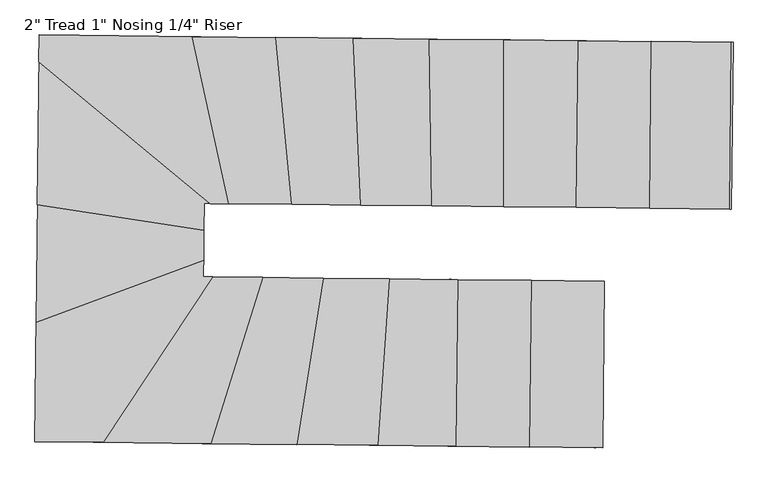
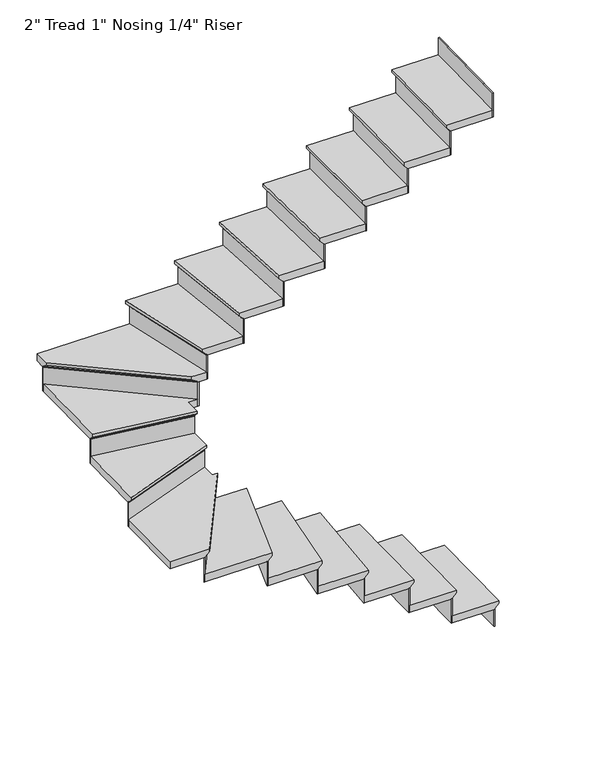
"""IFC4 building model written with IfcOpenShell, lengths in millimetres: stair flight geometry."""

from ifc_helpers import new_model, si_unit, origin, place, context, project, spatial, faceted_brep, source, transform, mapped, element, save


def stair_flight_e36c3716(model_context):
    return source(origin(), model_context, "Body", "Brep", [
        faceted_brep([(-1961.6349602, -4965.4067295, 9751.4833333), (-1961.6349602, -4965.4067295, 9770.5333333), (-1968.4523403, -5600.3701326, 9770.5333333), (-1968.4523403, -5600.3701326, 9751.4833333), (-1987.0334963, -4965.1340343, 9726.0833333), (-1993.8508764, -5600.0974374, 9726.0833333), (-2266.4173937, -4962.134387, 9770.5333333), (-2273.2347738, -5597.0977902, 9770.5333333), (-1993.8508764, -5600.0974374, 9719.7333333), (-2273.2347738, -5597.0977902, 9719.7333333), (-2266.4173937, -4962.134387, 9719.7333333), (-1987.0334963, -4965.1340343, 9719.7333333)], [[[0, 1, 2, 3]], [[4, 0, 3, 5]], [[2, 1, 6, 7]], [[8, 9, 10, 11]], [[2, 7, 9, 8, 5, 3]], [[8, 11, 4, 5]], [[6, 1, 0, 4, 11, 10]], [[7, 6, 10, 9]]]),
        faceted_brep([(-1987.0334963, -4965.1340343, 9719.7333333), (-1987.0334963, -4965.1340343, 9601.2), (-1993.3831304, -4965.0658605, 9601.2), (-1993.3831304, -4965.0658605, 9719.7333333), (-1993.8508764, -5600.0974374, 9719.7333333), (-2000.2005104, -5600.0292636, 9719.7333333), (-2000.2005104, -5600.0292636, 9601.2), (-1993.8508764, -5600.0974374, 9601.2)], [[[0, 1, 2, 3]], [[4, 5, 6, 7]], [[1, 0, 4, 7]], [[2, 1, 7, 6]], [[3, 2, 6, 5]], [[0, 3, 5, 4]]]),
        faceted_brep([(-2266.4173937, -4962.134387, 9889.0666667), (-2266.4173937, -4962.134387, 9719.7333333), (-2272.7670277, -4962.0662132, 9719.7333333), (-2272.7670277, -4962.0662132, 9889.0666667), (-2273.2347738, -5597.0977902, 9889.0666667), (-2279.5844078, -5597.0296164, 9889.0666667), (-2279.5844078, -5597.0296164, 9719.7333333), (-2273.2347738, -5597.0977902, 9719.7333333)], [[[0, 1, 2, 3]], [[4, 5, 6, 7]], [[1, 0, 4, 7]], [[2, 1, 7, 6]], [[3, 2, 6, 5]], [[0, 3, 5, 4]]]),
        faceted_brep([(-2247.8362377, -5597.3704854, 9939.8666667), (-2241.0188576, -4962.4070822, 9939.8666667), (-2545.8012911, -4959.1347398, 9939.8666667), (-2552.6186712, -5594.0981429, 9939.8666667), (-2273.2347738, -5597.0977902, 9889.0666667), (-2552.6186712, -5594.0981429, 9889.0666667), (-2545.8012911, -4959.1347398, 9889.0666667), (-2266.4173937, -4962.134387, 9889.0666667), (-2273.2347738, -5597.0977902, 9895.4166667), (-2247.8362377, -5597.3704854, 9920.8166667), (-2266.4173937, -4962.134387, 9895.4166667), (-2241.0188576, -4962.4070822, 9920.8166667)], [[[0, 1, 2, 3]], [[4, 5, 6, 7]], [[0, 3, 5, 4, 8, 9]], [[4, 7, 10, 8]], [[2, 1, 11, 10, 7, 6]], [[3, 2, 6, 5]], [[11, 1, 0, 9]], [[10, 11, 9, 8]]]),
        faceted_brep([(-2545.8012911, -4959.1347398, 10058.4), (-2545.8012911, -4959.1347398, 9889.0666667), (-2552.1509251, -4959.066566, 9889.0666667), (-2552.1509251, -4959.066566, 10058.4), (-2552.6186712, -5594.0981429, 10058.4), (-2558.9683052, -5594.0299691, 10058.4), (-2558.9683052, -5594.0299691, 9889.0666667), (-2552.6186712, -5594.0981429, 9889.0666667)], [[[0, 1, 2, 3]], [[4, 5, 6, 7]], [[1, 0, 4, 7]], [[2, 1, 7, 6]], [[3, 2, 6, 5]], [[0, 3, 5, 4]]]),
        faceted_brep([(-2527.2201351, -5594.3708381, 10109.2), (-2520.402755, -4959.407435, 10109.2), (-2806.7760852, -4956.3327447, 10109.2), (-2850.4973934, -5590.8999232, 10109.2), (-2552.6186712, -5594.0981429, 10058.4), (-2850.4973934, -5590.8999232, 10058.4), (-2806.7760852, -4956.3327447, 10058.4), (-2545.8012911, -4959.1347398, 10058.4), (-2552.6186712, -5594.0981429, 10064.75), (-2527.2201351, -5594.3708381, 10090.15), (-2545.8012911, -4959.1347398, 10064.75), (-2520.402755, -4959.407435, 10090.15)], [[[0, 1, 2, 3]], [[4, 5, 6, 7]], [[0, 3, 5, 4, 8, 9]], [[4, 7, 10, 8]], [[2, 1, 11, 10, 7, 6]], [[3, 2, 6, 5]], [[11, 1, 0, 9]], [[10, 11, 9, 8]]]),
        faceted_brep([(-2806.7760852, -4956.3327447, 10227.7333333), (-2806.7760852, -4956.3327447, 10058.4), (-2813.1364345, -4956.2644558, 10058.4), (-2813.1364345, -4956.2644558, 10227.7333333), (-2850.4973934, -5590.8999232, 10227.7333333), (-2856.8577426, -5590.8316344, 10227.7333333), (-2856.8577426, -5590.8316344, 10058.4), (-2850.4973934, -5590.8999232, 10058.4)], [[[0, 1, 2, 3]], [[4, 5, 6, 7]], [[1, 0, 4, 7]], [[2, 1, 7, 6]], [[3, 2, 6, 5]], [[0, 3, 5, 4]]]),
        faceted_brep([(-2825.0559965, -5591.1730786, 10278.5333333), (-2781.3346883, -4956.6059001, 10278.5333333), (-3058.0757112, -4953.6346284, 10278.5333333), (-3158.4280189, -5587.5937798, 10278.5333333), (-2850.4973934, -5590.8999232, 10227.7333333), (-3158.4280189, -5587.5937798, 10227.7333333), (-3058.0757112, -4953.6346284, 10227.7333333), (-2806.7760852, -4956.3327447, 10227.7333333), (-2850.4973934, -5590.8999232, 10234.0833333), (-2825.0559965, -5591.1730786, 10259.4833333), (-2806.7760852, -4956.3327447, 10234.0833333), (-2781.3346883, -4956.6059001, 10259.4833333)], [[[0, 1, 2, 3]], [[4, 5, 6, 7]], [[0, 3, 5, 4, 8, 9]], [[4, 7, 10, 8]], [[2, 1, 11, 10, 7, 6]], [[3, 2, 6, 5]], [[11, 1, 0, 9]], [[10, 11, 9, 8]]]),
        faceted_brep([(-3058.0757112, -4953.6346284, 10397.0666667), (-3058.0757112, -4953.6346284, 10227.7333333), (-3064.4938676, -4953.5657189, 10227.7333333), (-3064.4938676, -4953.5657189, 10397.0666667), (-3158.4280189, -5587.5937798, 10397.0666667), (-3164.8461752, -5587.5248703, 10397.0666667), (-3164.8461752, -5587.5248703, 10227.7333333), (-3158.4280189, -5587.5937798, 10227.7333333)], [[[0, 1, 2, 3]], [[4, 5, 6, 7]], [[1, 0, 4, 7]], [[2, 1, 7, 6]], [[3, 2, 6, 5]], [[0, 3, 5, 4]]]),
        faceted_brep([(-3132.7553936, -5587.8694178, 10447.8666667), (-3032.4030859, -4953.9102664, 10447.8666667), (-3289.3424431, -4951.1515984, 10447.8666667), (-3487.6403792, -5584.0591417, 10447.8666667), (-3158.4280189, -5587.5937798, 10397.0666667), (-3487.6403792, -5584.0591417, 10397.0666667), (-3289.3424431, -4951.1515984, 10397.0666667), (-3058.0757112, -4953.6346284, 10397.0666667), (-3158.4280189, -5587.5937798, 10403.4166667), (-3132.7553936, -5587.8694178, 10428.8166667), (-3058.0757112, -4953.6346284, 10403.4166667), (-3032.4030859, -4953.9102664, 10428.8166667)], [[[0, 1, 2, 3]], [[4, 5, 6, 7]], [[0, 3, 5, 4, 8, 9]], [[4, 7, 10, 8]], [[2, 1, 11, 10, 7, 6]], [[3, 2, 6, 5]], [[11, 1, 0, 9]], [[10, 11, 9, 8]]]),
        faceted_brep([(-3289.3424431, -4951.1515984, 10566.4), (-3289.3424431, -4951.1515984, 10397.0666667), (-3295.9745116, -4951.0803922, 10397.0666667), (-3295.9745116, -4951.0803922, 10566.4), (-3487.6403792, -5584.0591417, 10566.4), (-3494.2724477, -5583.9879355, 10566.4), (-3494.2724477, -5583.9879355, 10397.0666667), (-3487.6403792, -5584.0591417, 10397.0666667)], [[[0, 1, 2, 3]], [[4, 5, 6, 7]], [[1, 0, 4, 7]], [[2, 1, 7, 6]], [[3, 2, 6, 5]], [[0, 3, 5, 4]]]),
        faceted_brep([(-3461.1121052, -5584.3439665, 10617.2), (-3262.8141691, -4951.4364232, 10617.2), (-3484.2219113, -4949.0592457, 10617.2), (-3900.4163626, -5579.6273103, 10617.2), (-3487.6403792, -5584.0591417, 10566.4), (-3900.4163626, -5579.6273103, 10566.4), (-3484.2219113, -4949.0592457, 10566.4), (-3289.3424431, -4951.1515984, 10566.4), (-3487.6403792, -5584.0591417, 10572.75), (-3461.1121052, -5584.3439665, 10598.15), (-3289.3424431, -4951.1515984, 10572.75), (-3262.8141691, -4951.4364232, 10598.15)], [[[0, 1, 2, 3]], [[4, 5, 6, 7]], [[0, 3, 5, 4, 8, 9]], [[4, 7, 10, 8]], [[2, 1, 11, 10, 7, 6]], [[3, 2, 6, 5]], [[11, 1, 0, 9]], [[10, 11, 9, 8]]]),
        faceted_brep([(-3484.2219113, -4949.0592457, 10735.7333333), (-3484.2219113, -4949.0592457, 10566.4), (-3491.7768309, -4948.9781311, 10566.4), (-3491.7768309, -4948.9781311, 10735.7333333), (-3900.4163626, -5579.6273103, 10735.7333333), (-3907.9712823, -5579.5461958, 10735.7333333), (-3907.9712823, -5579.5461958, 10566.4), (-3900.4163626, -5579.6273103, 10566.4)], [[[0, 1, 2, 3]], [[4, 5, 6, 7]], [[1, 0, 4, 7]], [[2, 1, 7, 6]], [[3, 2, 6, 5]], [[0, 3, 5, 4]]]),
        faceted_brep([(-4125.8898698, -5095.6676694, 10786.5333333), (-4131.0593878, -5577.1509768, 10786.5333333), (-3870.196684, -5579.9517684, 10786.5333333), (-3454.0022327, -4949.3837038, 10786.5333333), (-3489.2786045, -4949.0049537, 10786.5333333), (-3488.312708, -4859.0423992, 10786.5333333), (-4131.0593878, -5577.1509768, 10735.7333333), (-4125.8898698, -5095.6676694, 10735.7333333), (-3488.312708, -4859.0423992, 10735.7333333), (-3489.2786045, -4949.0049537, 10735.7333333), (-3484.2219113, -4949.0592457, 10735.7333333), (-3900.4163626, -5579.6273103, 10735.7333333), (-3900.4163626, -5579.6273103, 10742.0833333), (-3870.196684, -5579.9517684, 10767.4833333), (-3484.2219113, -4949.0592457, 10742.0833333), (-3454.0022327, -4949.3837038, 10767.4833333)], [[[0, 1, 2, 3, 4, 5]], [[6, 7, 8, 9, 10, 11]], [[1, 0, 7, 6]], [[2, 1, 6, 11, 12, 13]], [[11, 10, 14, 12]], [[4, 3, 15, 14, 10, 9]], [[5, 4, 9, 8]], [[0, 5, 8, 7]], [[15, 3, 2, 13]], [[14, 15, 13, 12]]]),
        faceted_brep([(-3488.312708, -4859.0423992, 10905.0666667), (-3488.312708, -4859.0423992, 10735.7333333), (-3488.2396954, -4852.2420842, 10735.7333333), (-3488.2396954, -4852.2420842, 10905.0666667), (-4125.8898698, -5095.6676694, 10905.0666667), (-4125.8168572, -5088.8673543, 10905.0666667), (-4125.8168572, -5088.8673543, 10735.7333333), (-4125.8898698, -5095.6676694, 10735.7333333)], [[[0, 1, 2, 3]], [[4, 5, 6, 7]], [[1, 0, 4, 7]], [[2, 1, 7, 6]], [[3, 2, 6, 5]], [[0, 3, 5, 4]]]),
        faceted_brep([(-4126.1819202, -5122.8689296, 10955.8666667), (-3488.6047585, -4886.2436594, 10955.8666667), (-3487.1016265, -4746.243576, 10955.8666667), (-4121.0934321, -4648.9326558, 10955.8666667), (-4125.8898698, -5095.6676694, 10905.0666667), (-4121.0934321, -4648.9326558, 10905.0666667), (-3487.1016265, -4746.243576, 10905.0666667), (-3488.312708, -4859.0423992, 10905.0666667), (-4125.8898698, -5095.6676694, 10911.4166667), (-4126.1819202, -5122.8689296, 10936.8166667), (-3488.312708, -4859.0423992, 10911.4166667), (-3488.6047585, -4886.2436594, 10936.8166667)], [[[0, 1, 2, 3]], [[4, 5, 6, 7]], [[0, 3, 5, 4, 8, 9]], [[4, 7, 10, 8]], [[3, 2, 6, 5]], [[11, 1, 0, 9]], [[10, 11, 9, 8]], [[2, 1, 11, 10, 7, 6]]]),
        faceted_brep([(-3487.1016265, -4746.243576, 11074.4), (-3487.1016265, -4746.243576, 10905.0666667), (-3487.0327638, -4739.8297815, 10905.0666667), (-3487.0327638, -4739.8297815, 11074.4), (-4121.0934321, -4648.9326558, 11074.4), (-4121.0245695, -4642.5188612, 11074.4), (-4121.0245695, -4642.5188612, 10905.0666667), (-4121.0934321, -4648.9326558, 10905.0666667)], [[[0, 1, 2, 3]], [[4, 5, 6, 7]], [[1, 0, 4, 7]], [[2, 1, 7, 6]], [[3, 2, 6, 5]], [[0, 3, 5, 4]]]),
        faceted_brep([(-4121.3688828, -4674.587834, 11125.2), (-3487.3770772, -4771.8987542, 11125.2), (-3486.2789573, -4669.6210563, 11125.2), (-3423.6180491, -4670.2938246, 11125.2), (-4115.1699262, -4097.2237198, 11125.2), (-4121.0934321, -4648.9326558, 11074.4), (-4115.1699262, -4097.2237198, 11074.4), (-3423.6180491, -4670.2938246, 11074.4), (-3486.2789573, -4669.6210563, 11074.4), (-3487.1016265, -4746.243576, 11074.4), (-4121.0934321, -4648.9326558, 11080.75), (-4121.3688828, -4674.587834, 11106.15), (-3487.1016265, -4746.243576, 11080.75), (-3487.3770772, -4771.8987542, 11106.15)], [[[0, 1, 2, 3, 4]], [[5, 6, 7, 8, 9]], [[0, 4, 6, 5, 10, 11]], [[5, 9, 12, 10]], [[2, 1, 13, 12, 9, 8]], [[4, 3, 7, 6]], [[13, 1, 0, 11]], [[12, 13, 11, 10]], [[3, 2, 8, 7]]]),
        faceted_brep([(-3423.6180491, -4670.2938246, 11243.7333333), (-3423.6180491, -4670.2938246, 11074.4), (-3413.5354356, -4670.4020781, 11074.4), (-3413.5354356, -4670.4020781, 11243.7333333), (-4115.1699262, -4097.2237198, 11243.7333333), (-4115.0821626, -4089.0495147, 11243.7333333), (-4115.0821626, -4089.0495147, 11074.4), (-4115.1699262, -4097.2237198, 11074.4)], [[[0, 1, 2, 3]], [[4, 5, 6, 7]], [[1, 0, 4, 7]], [[2, 1, 7, 6]], [[3, 2, 6, 5]], [[0, 3, 5, 4]]]),
        faceted_brep([(-3506.4342514, -4034.368057, 11294.5333333), (-4114.4249804, -4027.8402731, 11294.5333333), (-4115.5209805, -4129.9205399, 11294.5333333), (-3463.9485035, -4669.8608106, 11294.5333333), (-3365.8789969, -4670.9137486, 11294.5333333), (-4114.4249804, -4027.8402731, 11243.7333333), (-3506.4342514, -4034.368057, 11243.7333333), (-3365.8789969, -4670.9137486, 11243.7333333), (-3423.6180491, -4670.2938246, 11243.7333333), (-4115.1699262, -4097.2237198, 11243.7333333), (-3423.6180491, -4670.2938246, 11250.0833333), (-4115.1699262, -4097.2237198, 11250.0833333), (-3463.9485035, -4669.8608106, 11275.4833333), (-4115.5209805, -4129.9205399, 11275.4833333)], [[[0, 1, 2, 3, 4]], [[5, 6, 7, 8, 9]], [[1, 0, 6, 5]], [[9, 8, 10, 11]], [[4, 3, 12, 10, 8, 7]], [[0, 4, 7, 6]], [[12, 3, 2, 13]], [[10, 12, 13, 11]], [[2, 1, 5, 9, 11, 13]]]),
        faceted_brep([(-3365.8789969, -4670.9137486, 11413.0666667), (-3365.8789969, -4670.9137486, 11243.7333333), (-3359.3605829, -4670.9837346, 11243.7333333), (-3359.3605829, -4670.9837346, 11413.0666667), (-3506.4342514, -4034.368057, 11413.0666667), (-3499.9158374, -4034.438043, 11413.0666667), (-3499.9158374, -4034.438043, 11243.7333333), (-3506.4342514, -4034.368057, 11243.7333333)], [[[0, 1, 2, 3]], [[4, 5, 6, 7]], [[1, 0, 4, 7]], [[2, 1, 7, 6]], [[3, 2, 6, 5]], [[0, 3, 5, 4]]]),
        faceted_brep([(-3532.5079076, -4034.0881133, 11463.8666667), (-3391.9526531, -4670.6338049, 11463.8666667), (-3127.2086135, -4673.4762691, 11463.8666667), (-3187.4049598, -4037.793363, 11463.8666667), (-3506.4342514, -4034.368057, 11413.0666667), (-3187.4049598, -4037.793363, 11413.0666667), (-3127.2086135, -4673.4762691, 11413.0666667), (-3365.8789969, -4670.9137486, 11413.0666667), (-3506.4342514, -4034.368057, 11419.4166667), (-3532.5079076, -4034.0881133, 11444.8166667), (-3365.8789969, -4670.9137486, 11419.4166667), (-3391.9526531, -4670.6338049, 11444.8166667)], [[[0, 1, 2, 3]], [[4, 5, 6, 7]], [[0, 3, 5, 4, 8, 9]], [[4, 7, 10, 8]], [[2, 1, 11, 10, 7, 6]], [[3, 2, 6, 5]], [[11, 1, 0, 9]], [[10, 11, 9, 8]]]),
        faceted_brep([(-3127.2086135, -4673.4762691, 11582.4), (-3127.2086135, -4673.4762691, 11413.0666667), (-3120.8237144, -4673.5448215, 11413.0666667), (-3120.8237144, -4673.5448215, 11582.4), (-3187.4049598, -4037.793363, 11582.4), (-3181.0200608, -4037.8619154, 11582.4), (-3181.0200608, -4037.8619154, 11413.0666667), (-3187.4049598, -4037.793363, 11413.0666667)], [[[0, 1, 2, 3]], [[4, 5, 6, 7]], [[1, 0, 4, 7]], [[2, 1, 7, 6]], [[3, 2, 6, 5]], [[0, 3, 5, 4]]]),
        faceted_brep([(-3212.9445562, -4037.5191533, 11633.2), (-3152.7482098, -4673.2020594, 11633.2), (-2863.8799111, -4676.3035373, 11633.2), (-2892.1704009, -4040.9631932, 11633.2), (-3187.4049598, -4037.793363, 11582.4), (-2892.1704009, -4040.9631932, 11582.4), (-2863.8799111, -4676.3035373, 11582.4), (-3127.2086135, -4673.4762691, 11582.4), (-3187.4049598, -4037.793363, 11588.75), (-3212.9445562, -4037.5191533, 11614.15), (-3127.2086135, -4673.4762691, 11588.75), (-3152.7482098, -4673.2020594, 11614.15)], [[[0, 1, 2, 3]], [[4, 5, 6, 7]], [[0, 3, 5, 4, 8, 9]], [[4, 7, 10, 8]], [[2, 1, 11, 10, 7, 6]], [[3, 2, 6, 5]], [[11, 1, 0, 9]], [[10, 11, 9, 8]]]),
        faceted_brep([(-2863.8799111, -4676.3035373, 11751.7333333), (-2863.8799111, -4676.3035373, 11582.4), (-2857.5205787, -4676.3718152, 11582.4), (-2857.5205787, -4676.3718152, 11751.7333333), (-2892.1704009, -4040.9631932, 11751.7333333), (-2885.8110685, -4041.0314712, 11751.7333333), (-2885.8110685, -4041.0314712, 11582.4), (-2892.1704009, -4040.9631932, 11582.4)], [[[0, 1, 2, 3]], [[4, 5, 6, 7]], [[1, 0, 4, 7]], [[2, 1, 7, 6]], [[3, 2, 6, 5]], [[0, 3, 5, 4]]]),
        faceted_brep([(-2917.6077305, -4040.6900815, 11802.5333333), (-2889.3172407, -4676.0304256, 11802.5333333), (-2593.0867697, -4679.2109486, 11802.5333333), (-2604.2529652, -4044.0544621, 11802.5333333), (-2892.1704009, -4040.9631932, 11751.7333333), (-2604.2529652, -4044.0544621, 11751.7333333), (-2593.0867697, -4679.2109486, 11751.7333333), (-2863.8799111, -4676.3035373, 11751.7333333), (-2892.1704009, -4040.9631932, 11758.0833333), (-2917.6077305, -4040.6900815, 11783.4833333), (-2863.8799111, -4676.3035373, 11758.0833333), (-2889.3172407, -4676.0304256, 11783.4833333)], [[[0, 1, 2, 3]], [[4, 5, 6, 7]], [[0, 3, 5, 4, 8, 9]], [[4, 7, 10, 8]], [[2, 1, 11, 10, 7, 6]], [[3, 2, 6, 5]], [[11, 1, 0, 9]], [[10, 11, 9, 8]]]),
        faceted_brep([(-2593.0867697, -4679.2109486, 11921.0666667), (-2593.0867697, -4679.2109486, 11751.7333333), (-2586.7345895, -4679.2791497, 11751.7333333), (-2586.7345895, -4679.2791497, 11921.0666667), (-2604.2529652, -4044.0544621, 11921.0666667), (-2597.900785, -4044.1226632, 11921.0666667), (-2597.900785, -4044.1226632, 11751.7333333), (-2604.2529652, -4044.0544621, 11751.7333333)], [[[0, 1, 2, 3]], [[4, 5, 6, 7]], [[1, 0, 4, 7]], [[2, 1, 7, 6]], [[3, 2, 6, 5]], [[0, 3, 5, 4]]]),
        faceted_brep([(-2629.661686, -4043.7816575, 11971.8666667), (-2618.4954904, -4678.9381441, 11971.8666667), (-2319.0528449, -4682.1531551, 11971.8666667), (-2319.536107, -4047.1113675, 11971.8666667), (-2604.2529652, -4044.0544621, 11921.0666667), (-2319.536107, -4047.1113675, 11921.0666667), (-2319.0528449, -4682.1531551, 11921.0666667), (-2593.0867697, -4679.2109486, 11921.0666667), (-2604.2529652, -4044.0544621, 11927.4166667), (-2629.661686, -4043.7816575, 11952.8166667), (-2593.0867697, -4679.2109486, 11927.4166667), (-2618.4954904, -4678.9381441, 11952.8166667)], [[[0, 1, 2, 3]], [[4, 5, 6, 7]], [[0, 3, 5, 4, 8, 9]], [[4, 7, 10, 8]], [[2, 1, 11, 10, 7, 6]], [[3, 2, 6, 5]], [[11, 1, 0, 9]], [[10, 11, 9, 8]]]),
        faceted_brep([(-2319.0528449, -4682.1531551, 12090.4), (-2319.0528449, -4682.1531551, 11921.0666667), (-2312.7027912, -4682.2213334, 11921.0666667), (-2312.7027912, -4682.2213334, 12090.4), (-2319.536107, -4047.1113675, 12090.4), (-2313.1860533, -4047.1795458, 12090.4), (-2313.1860533, -4047.1795458, 11921.0666667), (-2319.536107, -4047.1113675, 11921.0666667)], [[[0, 1, 2, 3]], [[4, 5, 6, 7]], [[1, 0, 4, 7]], [[2, 1, 7, 6]], [[3, 2, 6, 5]], [[0, 3, 5, 4]]]),
        faceted_brep([(-2344.9363219, -4046.8386542, 12141.2), (-2344.4530598, -4681.8804418, 12141.2), (-2043.3209474, -4685.113592, 12141.2), (-2036.5035673, -4050.1501889, 12141.2), (-2319.536107, -4047.1113675, 12090.4), (-2036.5035673, -4050.1501889, 12090.4), (-2043.3209474, -4685.113592, 12090.4), (-2319.0528449, -4682.1531551, 12090.4), (-2319.536107, -4047.1113675, 12096.75), (-2344.9363219, -4046.8386542, 12122.15), (-2319.0528449, -4682.1531551, 12096.75), (-2344.4530598, -4681.8804418, 12122.15)], [[[0, 1, 2, 3]], [[4, 5, 6, 7]], [[0, 3, 5, 4, 8, 9]], [[4, 7, 10, 8]], [[2, 1, 11, 10, 7, 6]], [[3, 2, 6, 5]], [[11, 1, 0, 9]], [[10, 11, 9, 8]]]),
        faceted_brep([(-2043.3209474, -4685.113592, 12259.7333333), (-2043.3209474, -4685.113592, 12090.4), (-2036.9713133, -4685.1817658, 12090.4), (-2036.9713133, -4685.1817658, 12259.7333333), (-2036.5035673, -4050.1501889, 12259.7333333), (-2030.1539332, -4050.2183627, 12259.7333333), (-2030.1539332, -4050.2183627, 12090.4), (-2036.5035673, -4050.1501889, 12090.4)], [[[0, 1, 2, 3]], [[4, 5, 6, 7]], [[1, 0, 4, 7]], [[2, 1, 7, 6]], [[3, 2, 6, 5]], [[0, 3, 5, 4]]]),
        faceted_brep([(-2061.9021034, -4049.8774937, 12310.5333333), (-2068.7194835, -4684.8408968, 12310.5333333), (-1763.93705, -4688.1132393, 12310.5333333), (-1757.1196699, -4053.1498361, 12310.5333333), (-2036.5035673, -4050.1501889, 12259.7333333), (-1757.1196699, -4053.1498361, 12259.7333333), (-1763.93705, -4688.1132393, 12259.7333333), (-2043.3209474, -4685.113592, 12259.7333333), (-2036.5035673, -4050.1501889, 12266.0833333), (-2061.9021034, -4049.8774937, 12291.4833333), (-2043.3209474, -4685.113592, 12266.0833333), (-2068.7194835, -4684.8408968, 12291.4833333)], [[[0, 1, 2, 3]], [[4, 5, 6, 7]], [[0, 3, 5, 4, 8, 9]], [[4, 7, 10, 8]], [[2, 1, 11, 10, 7, 6]], [[3, 2, 6, 5]], [[11, 1, 0, 9]], [[10, 11, 9, 8]]]),
        faceted_brep([(-1763.93705, -4688.1132393, 12429.0666667), (-1763.93705, -4688.1132393, 12259.7333333), (-1757.5874159, -4688.1814131, 12259.7333333), (-1757.5874159, -4688.1814131, 12429.0666667), (-1757.1196699, -4053.1498361, 12429.0666667), (-1750.7700359, -4053.2180099, 12429.0666667), (-1750.7700359, -4053.2180099, 12259.7333333), (-1757.1196699, -4053.1498361, 12259.7333333)], [[[0, 1, 2, 3]], [[4, 5, 6, 7]], [[1, 0, 4, 7]], [[2, 1, 7, 6]], [[3, 2, 6, 5]], [[0, 3, 5, 4]]]),
        faceted_brep([(-1484.5531526, -4691.1128865, 12598.4), (-1484.5531526, -4691.1128865, 12429.0666667), (-1478.2035186, -4691.1810603, 12429.0666667), (-1478.2035186, -4691.1810603, 12598.4), (-1477.7357725, -4056.1494834, 12598.4), (-1471.3861385, -4056.2176572, 12598.4), (-1471.3861385, -4056.2176572, 12429.0666667), (-1477.7357725, -4056.1494834, 12429.0666667)], [[[0, 1, 2, 3]], [[4, 5, 6, 7]], [[1, 0, 4, 7]], [[2, 1, 7, 6]], [[3, 2, 6, 5]], [[0, 3, 5, 4]]]),
        faceted_brep([(-1782.518206, -4052.8771409, 12479.8666667), (-1789.3355861, -4687.8405441, 12479.8666667), (-1484.5531526, -4691.1128865, 12479.8666667), (-1477.7357725, -4056.1494834, 12479.8666667), (-1757.1196699, -4053.1498361, 12429.0666667), (-1477.7357725, -4056.1494834, 12429.0666667), (-1484.5531526, -4691.1128865, 12429.0666667), (-1763.93705, -4688.1132393, 12429.0666667), (-1757.1196699, -4053.1498361, 12435.4166667), (-1782.518206, -4052.8771409, 12460.8166667), (-1763.93705, -4688.1132393, 12435.4166667), (-1789.3355861, -4687.8405441, 12460.8166667)], [[[0, 1, 2, 3]], [[4, 5, 6, 7]], [[0, 3, 5, 4, 8, 9]], [[4, 7, 10, 8]], [[2, 1, 11, 10, 7, 6]], [[3, 2, 6, 5]], [[11, 1, 0, 9]], [[10, 11, 9, 8]]]),
    ])


if __name__ == "__main__":
    model = new_model("IFC4")
    model_context = context("Model", 3, world=origin())
    ifc_project = project(units=[si_unit("LENGTHUNIT", "METRE", prefix="MILLI")], contexts=[model_context])
    site = spatial("IfcSite", under=ifc_project)
    building = spatial("IfcBuilding", under=site)
    placement = place(None, origin())
    stair_flight_shape = stair_flight_e36c3716(model_context)
    element("IfcStairFlight", 1, ObjectType="2\" Tread 1\" Nosing 1/4\" Riser", at=placement, inside=building, context=model_context, shape_type="MappedRepresentation", body=[
        mapped(stair_flight_shape, transform((0.0, 0.0, 0.0), x_axis=(1.0, 0.0, 0.0), y_axis=(0.0, 1.0, 0.0), z_axis=(0.0, 0.0, 1.0))),
    ])
    save(model, "model.ifc")
